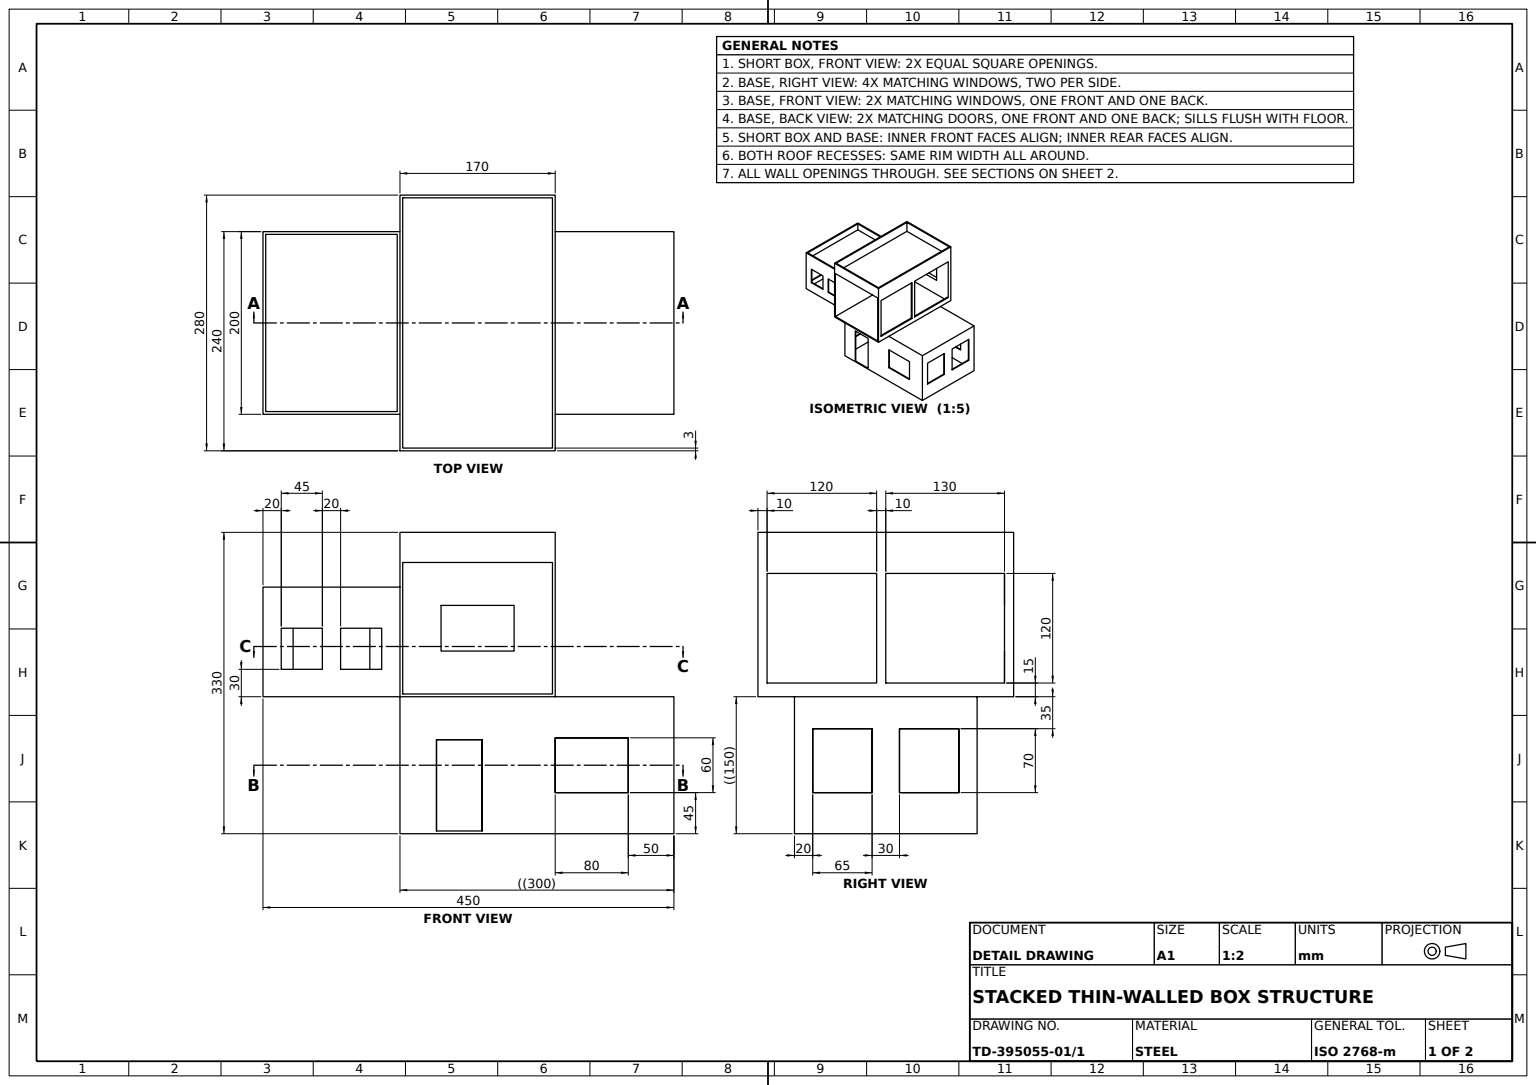
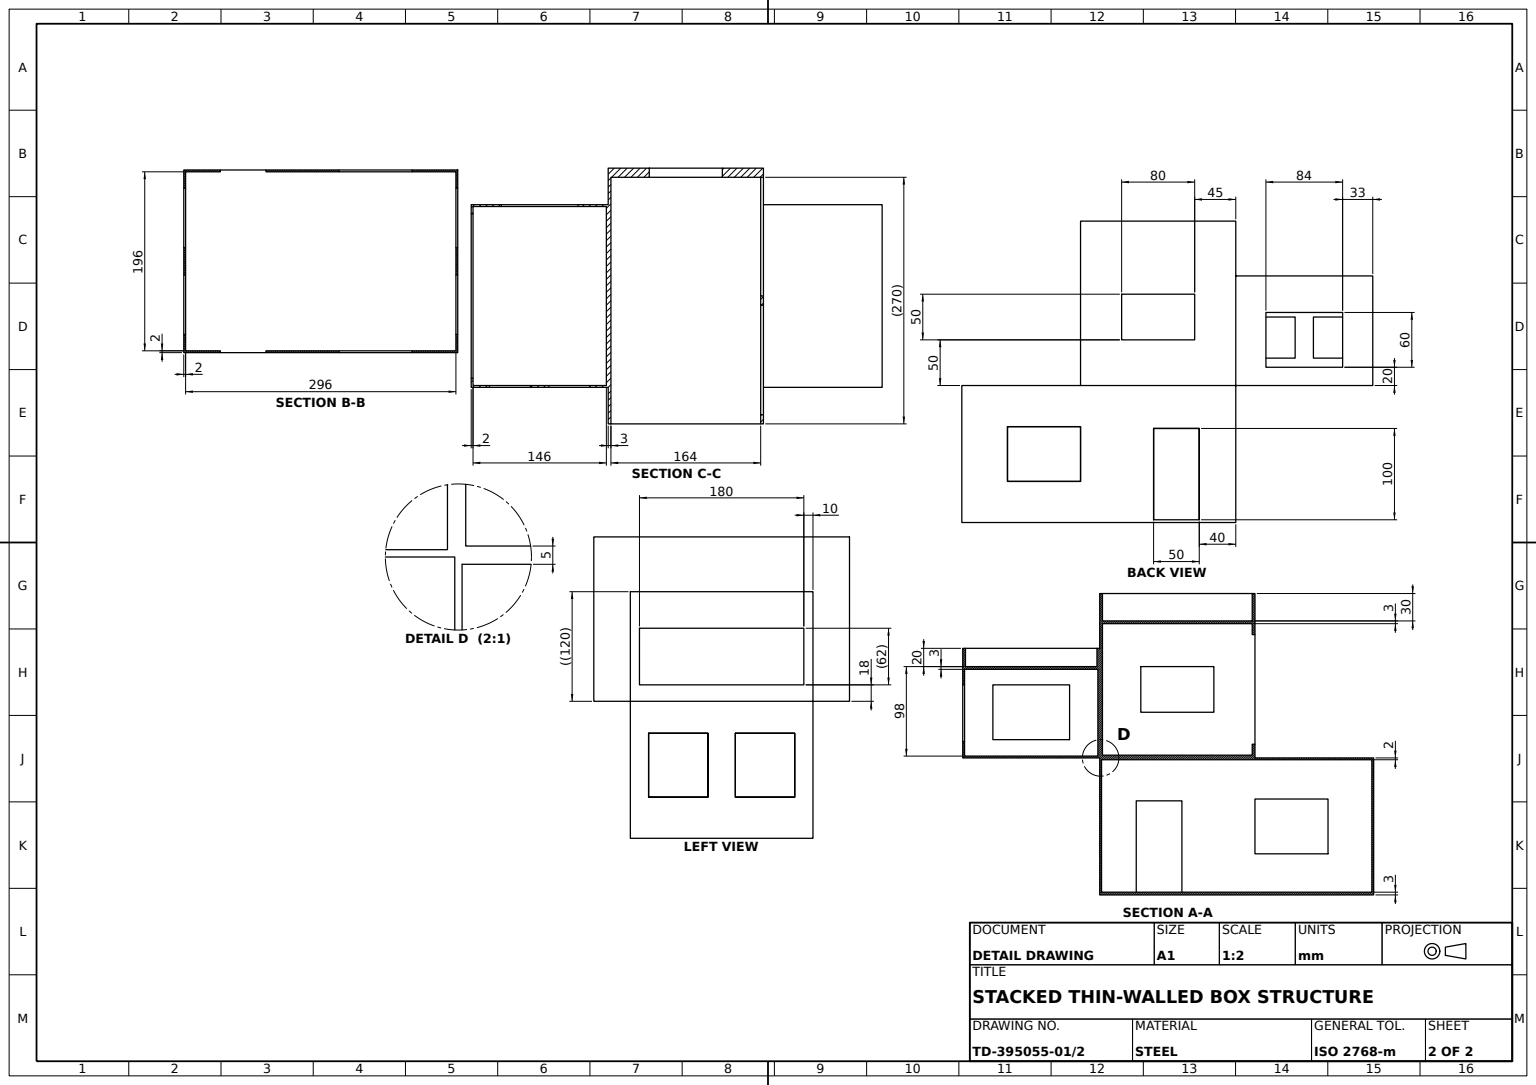
SolidWorks part; units mm, degrees
material "Plain Carbon Steel"
ref_plane "Front Plane" through (0, 0, 0) normal (0, 0, 1) x (1, 0, 0)
ref_plane "Top Plane" through (0, 0, 0) normal (0, 1, 0) x (1, 0, 0)
ref_plane "Right Plane" through (0, 0, 0) normal (1, 0, 0) x (0, 0, -1)
sketch "Ground Floor Footprint Sketch" plane through (0, 0, 0) normal (0, 1, 0) x (1, 0, 0)
  line L1 (0, 0) -> (300, 0)
  line L2 (0, 0) -> (0, 200)
  line L3 (0, 200) -> (300, 200)
  line L4 (300, 0) -> (300, 200)
  dimension "D1" = 300
  dimension "D2" = 200
extrude "Ground Floor Block" add sketch "Ground Floor Footprint Sketch" along normal blind 150
sketch "Ground Floor Door Sketch" plane through (0, 0, 0) normal (0, 0, 1) x (1, 0, 0)
  line L1 (40, 3) -> (90, 3)
  line L2 (40, 3) -> (40, 103)
  line L3 (40, 103) -> (90, 103)
  line L4 (90, 3) -> (90, 103)
  dimension "D1" = 3
  dimension "D2" = 40
  dimension "D3" = 100
  dimension "D4" = 50
extrude "Ground Floor Door Opening" cut sketch "Ground Floor Door Sketch" against normal blind 210
sketch "Ground Floor Interior Sketch" plane through (0, 150, 0) normal (0, 1, 0) x (1, 0, 0)
  line L0 (0, 0) -> (300, 0) construction
  line L1 (2, 198) -> (298, 198)
  line L2 (2, 198) -> (2, 2)
  line L3 (2, 2) -> (298, 2)
  line L4 (298, 198) -> (298, 2)
  line L5 (0, 200) -> (0, 0) construction
  line L6 (300, 0) -> (300, 200) construction
  line L7 (300, 200) -> (0, 200) construction
  dimension "D1" = 2
  dimension "D2" = 2
  dimension "D3" = 2
  dimension "D4" = 2
extrude "Ground Floor Interior Pocket" cut sketch "Ground Floor Interior Sketch" against normal up to surface (147 mm away) up to face at (65, 3, -100)
sketch "Ground Floor Slab Sketch" plane through (0, 150, 0) normal (0, 1, 0) x (1, 0, 0)
  line L1 (0, 200) -> (300, 200)
  line L2 (0, 200) -> (0, 0)
  line L3 (0, 0) -> (300, 0)
  line L4 (300, 200) -> (300, 0)
extrude "Ground Floor Slab" add sketch "Ground Floor Slab Sketch" against normal blind 2
sketch "Ground Floor Window Sketch" plane through (0, 0, 0) normal (0, 0, 1) x (1, 0, 0)
  line L1 (170, 105) -> (250, 105)
  line L2 (170, 105) -> (170, 45)
  line L3 (170, 45) -> (250, 45)
  line L4 (250, 105) -> (250, 45)
  dimension "D1" = 45
  dimension "D2" = 45
  dimension "D3" = 80
  dimension "D4" = 50
extrude "Ground Floor Window" cut sketch "Ground Floor Window Sketch" against normal blind 312
sketch "Ground Floor Side Windows Sketch" plane through (300, 0, 0) normal (1, 0, 0) x (0, 0, -1)
  line L1 (20, 45) -> (85, 45)
  line L2 (20, 45) -> (20, 115)
  line L3 (20, 115) -> (85, 115)
  line L4 (85, 45) -> (85, 115)
  line L5 (115, 45) -> (180, 45)
  line L6 (115, 45) -> (115, 115)
  line L7 (115, 115) -> (180, 115)
  line L8 (180, 45) -> (180, 115)
  dimension "D1" = 20
  dimension "D2" = 20
  dimension "D3" = 65
  dimension "D4" = 65
  dimension "D5" = 45
  dimension "D6" = 70
  dimension "D7" = 45
  dimension "D8" = 70
extrude "Ground Floor Side Windows" cut sketch "Ground Floor Side Windows Sketch" against normal blind 312
sketch "First Floor Footprint Sketch" plane through (0, 150, 0) normal (0, 1, 0) x (1, 0, 0)
  line L1 (0, 0) -> (-150, 0)
  line L2 (0, 0) -> (0, 200)
  line L3 (0, 200) -> (-150, 200)
  line L4 (-150, 0) -> (-150, 200)
  dimension "D1" = 200
  dimension "D2" = 150
extrude "First Floor Block" add sketch "First Floor Footprint Sketch" along normal blind 100 separate body
sketch "First Floor Interior Sketch" plane through (0, 250, 0) normal (0, 1, 0) x (1, 0, 0)
  line L0 (-150, 0) -> (0, 0) construction
  line L1 (-148, 198) -> (-2, 198)
  line L2 (-148, 198) -> (-148, 2)
  line L3 (-148, 2) -> (-2, 2)
  line L4 (-2, 198) -> (-2, 2)
  line L5 (-150, 200) -> (-150, 0) construction
  line L6 (0, 0) -> (0, 200) construction
  line L7 (0, 200) -> (-150, 200) construction
  dimension "D1" = 2
  dimension "D2" = 2
  dimension "D3" = 2
  dimension "D4" = 2
extrude "First Floor Interior Pocket" cut sketch "First Floor Interior Sketch" against normal blind 98
sketch "First Floor Slab Sketch" plane through (0, 250, 0) normal (0, 1, 0) x (1, 0, 0)
  line L1 (-150, 200) -> (0, 200)
  line L2 (-150, 200) -> (-150, 0)
  line L3 (-150, 0) -> (0, 0)
  line L4 (0, 200) -> (0, 0)
extrude "First Floor Slab" add sketch "First Floor Slab Sketch" against normal blind 3
sketch "First Floor Door Sketch" plane through (-150, 0, 0) normal (-1, 0, 0) x (0, 0, 1)
  line L0 (-200, 150) -> (0, 150) construction
  line L1 (-190, 168) -> (-10, 168)
  line L2 (-190, 168) -> (-190, 230)
  line L3 (-190, 230) -> (-10, 230)
  line L4 (-10, 168) -> (-10, 230)
  line L5 (0, 250) -> (0, 150) construction
  line L6 (-200, 250) -> (-200, 150) construction
  dimension "D1" = 18
  dimension "D2" = 10
  dimension "D3" = 10
  dimension "D4" = 20
extrude "First Floor Door Opening" cut sketch "First Floor Door Sketch" against normal blind 23
sketch "First Floor Twin Windows Sketch" plane through (0, 0, 0) normal (0, 0, 1) x (1, 0, 0)
  line L1 (-130, 225) -> (-85, 225)
  line L2 (-130, 225) -> (-130, 180)
  line L3 (-130, 180) -> (-85, 180)
  line L4 (-85, 225) -> (-85, 180)
  line L5 (-65, 225) -> (-20, 225)
  line L6 (-65, 225) -> (-65, 180)
  line L7 (-65, 180) -> (-20, 180)
  line L8 (-20, 225) -> (-20, 180)
  dimension "D1" = 20
  dimension "D2" = 20
  dimension "D3" = 45
  dimension "D4" = 45
  dimension "D5" = 45
  dimension "D6" = 45
  dimension "D7" = 30
  dimension "D8" = 30
extrude "First Floor Twin Windows" cut sketch "First Floor Twin Windows Sketch" against normal blind 23
sketch "First Floor Window Sketch" plane through (0, 0, -200) normal (0, 0, -1) x (-1, 0, 0)
  line L1 (117, 170) -> (33, 170)
  line L2 (117, 170) -> (117, 230)
  line L3 (117, 230) -> (33, 230)
  line L4 (33, 170) -> (33, 230)
  dimension "D1" = 33
  dimension "D2" = 33
  dimension "D3" = 60
  dimension "D4" = 20
extrude "First Floor Window" cut sketch "First Floor Window Sketch" against normal blind 23
sketch "First Floor Parapet Front Sketch" plane through (-150, 0, 0) normal (-1, 0, 0) x (0, 0, 1)
  line L1 (-200, 250) -> (0, 250)
  line L2 (-200, 250) -> (-200, 270)
  line L3 (-200, 270) -> (0, 270)
  line L4 (0, 250) -> (0, 270)
  dimension "D1" = 20
  dimension "D2" = 200
extrude "First Floor Parapet Front" add sketch "First Floor Parapet Front Sketch" against normal blind 3
sketch "First Floor Parapet Side 1 Sketch" plane through (0, 0, -200) normal (0, 0, -1) x (-1, 0, 0)
  line L1 (0, 250) -> (150, 250)
  line L2 (0, 250) -> (0, 270)
  line L3 (0, 270) -> (150, 270)
  line L4 (150, 250) -> (150, 270)
extrude "First Floor Parapet Side 1" add sketch "First Floor Parapet Side 1 Sketch" against normal blind 3
sketch "First Floor Parapet Side 2 Sketch" plane through (0, 0, 0) normal (0, 0, 1) x (1, 0, 0)
  line L1 (0, 250) -> (-150, 250)
  line L2 (0, 250) -> (0, 270)
  line L3 (0, 270) -> (-150, 270)
  line L4 (-150, 250) -> (-150, 270)
extrude "First Floor Parapet Side 2" add sketch "First Floor Parapet Side 2 Sketch" against normal blind 3
sketch "First Floor Parapet Rear Sketch" plane through (0, 0, 0) normal (1, 0, 0) x (0, 0, -1)
  line L0 (197, 270) -> (197, 250) construction
  line L1 (0, 270) -> (197, 270)
  line L2 (0, 270) -> (0, 250)
  line L3 (0, 250) -> (197, 250)
  line L4 (197, 270) -> (197, 250)
  line L5 (197, 250) -> (3, 250) construction
extrude "First Floor Parapet Rear" add sketch "First Floor Parapet Rear Sketch" against normal blind 3
sketch "Upper Floor Profile Sketch" plane through (0, 0, 0) normal (0, 0, 1) x (1, 0, 0)
  line L1 (0, 150) -> (170, 150)
  line L2 (0, 150) -> (0, 300)
  line L3 (0, 300) -> (170, 300)
  line L4 (170, 150) -> (170, 300)
  dimension "D1" = 170
  dimension "D2" = 150
extrude "Upper Floor Block" add sketch "Upper Floor Profile Sketch" against normal blind 240 and the other way blind 40
sketch "Upper Floor Interior Sketch" plane through (0, 0, 40) normal (0, 0, 1) x (1, 0, 0)
  line L0 (0, 150) -> (170, 150) construction
  line L1 (3, 153) -> (167, 153)
  line L2 (3, 153) -> (3, 297)
  line L3 (3, 297) -> (167, 297)
  line L4 (167, 153) -> (167, 297)
  line L5 (170, 150) -> (170, 300) construction
  line L6 (170, 300) -> (0, 300) construction
  line L7 (0, 300) -> (0, 150) construction
  dimension "D1" = 3
  dimension "D2" = 3
  dimension "D3" = 3
  dimension "D4" = 3
extrude "Upper Floor Interior Pocket" cut sketch "Upper Floor Interior Sketch" against normal blind 270
sketch "Upper Floor Opening 1 Sketch" plane through (170, 0, 0) normal (1, 0, 0) x (0, 0, -1)
  line L1 (-30, 165) -> (90, 165)
  line L2 (-30, 165) -> (-30, 285)
  line L3 (-30, 285) -> (90, 285)
  line L4 (90, 165) -> (90, 285)
  dimension "D1" = 15
  dimension "D2" = 120
  dimension "D3" = 10
  dimension "D4" = 120
extrude "Upper Floor Opening 1" cut sketch "Upper Floor Opening 1 Sketch" against normal blind 100
sketch "Upper Floor Opening 2 Sketch" plane through (170, 0, 0) normal (1, 0, 0) x (0, 0, -1)
  line L1 (100, 285) -> (230, 285)
  line L2 (100, 285) -> (100, 165)
  line L3 (100, 165) -> (230, 165)
  line L4 (230, 285) -> (230, 165)
  dimension "D1" = 10
  dimension "D2" = 10
  dimension "D3" = 15
  dimension "D4" = 120
extrude "Upper Floor Opening 2" cut sketch "Upper Floor Opening 2 Sketch" against normal blind 100
sketch "Upper Floor Window Sketch" plane through (0, 0, -240) normal (0, 0, -1) x (-1, 0, 0)
  line L1 (-125, 250) -> (-45, 250)
  line L2 (-125, 250) -> (-125, 200)
  line L3 (-125, 200) -> (-45, 200)
  line L4 (-45, 250) -> (-45, 200)
  dimension "D1" = 50
  dimension "D2" = 50
  dimension "D3" = 80
  dimension "5" = 45
extrude "Upper Floor Window" cut sketch "Upper Floor Window Sketch" against normal blind 100
sketch "Upper Floor Parapet Front Sketch" plane through (0, 0, -240) normal (0, 0, -1) x (-1, 0, 0)
  line L1 (-170, 300) -> (0, 300)
  line L2 (-170, 300) -> (-170, 330)
  line L3 (-170, 330) -> (0, 330)
  line L4 (0, 300) -> (0, 330)
  dimension "D1" = 30
  dimension "D2" = 170
extrude "Upper Floor Parapet Front" add sketch "Upper Floor Parapet Front Sketch" against normal blind 3
sketch "Upper Floor Parapet Side 1 Sketch" plane through (170, 0, 0) normal (1, 0, 0) x (0, 0, -1)
  line L0 (-40, 150) -> (-40, 300) construction
  line L1 (237, 300) -> (-40, 300)
  line L2 (237, 300) -> (237, 330)
  line L3 (237, 330) -> (-40, 330)
  line L4 (-40, 300) -> (-40, 330)
  dimension "D1" = 30
extrude "Upper Floor Parapet Side 1" add sketch "Upper Floor Parapet Side 1 Sketch" against normal blind 3
sketch "Upper Floor Parapet Side 2 Sketch" plane through (0, 0, 40) normal (0, 0, 1) x (1, 0, 0)
  line L1 (0, 300) -> (170, 300)
  line L2 (0, 300) -> (0, 330)
  line L3 (0, 330) -> (170, 330)
  line L4 (170, 300) -> (170, 330)
extrude "Upper Floor Parapet Side 2" add sketch "Upper Floor Parapet Side 2 Sketch" against normal blind 3
sketch "Upper Floor Parapet Rear Sketch" plane through (0, 0, 0) normal (-1, 0, 0) x (0, 0, 1)
  line L1 (-237, 300) -> (37, 300)
  line L2 (-237, 300) -> (-237, 330)
  line L3 (-237, 330) -> (37, 330)
  line L4 (37, 300) -> (37, 330)
extrude "Upper Floor Parapet Rear" add sketch "Upper Floor Parapet Rear Sketch" against normal blind 3
